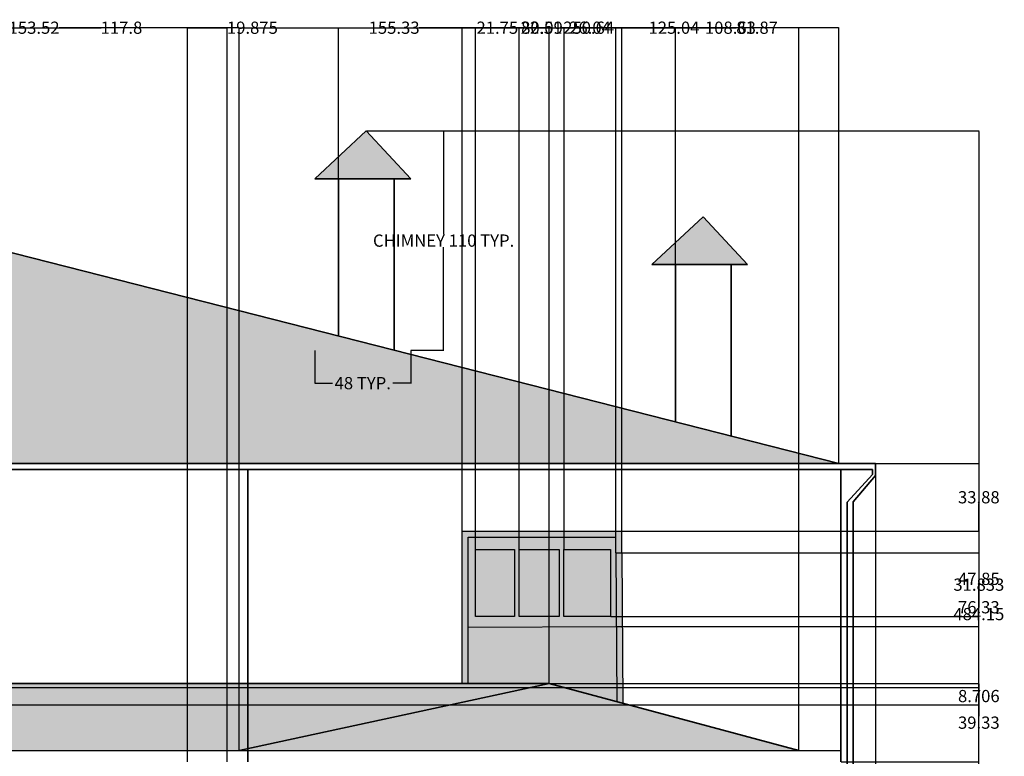
# Model space of a CAD drawing. Units: inches. Extents: x -655 to 499, y 20 to 616.
# Tile 7 of 7: x 5 to 499, y 246 to 616. Entities that reach past the tile are written whole.
import ezdxf

# ---------------------------------------------------------------- set-up
doc = ezdxf.new("R2010")
doc.units = ezdxf.units.IN
doc.header["$MEASUREMENT"] = 0
for name, color, linetype, lineweight in [('A-ANNO-DIMS', 2, 'Continuous', 18), ('A-ELEV', 7, 'Continuous', 35), ('A-ELEV-PATT', 9, 'Continuous', 13), ('A-GLAZ', 3, 'Continuous', 25), ('A-ROOF', 1, 'Continuous', 35)]:
    doc.layers.add(name, color=color, linetype=linetype, lineweight=lineweight)
doc.styles.get("Standard").update_dxf_attribs({"font": 'arial.ttf'})
doc.dimstyles.get("Standard").update_dxf_attribs({"dimtxt": 6.125, "dimasz": 0.18, "dimexe": 0.18, "dimexo": 0.0625, "dimgap": 0.09, "dimtad": 0, "dimtih": 1, "dimtoh": 1, "dimdec": 4, "dimzin": 0, "dimdsep": 46, "dimlunit": 4, "dimtxsty": 'Standard', "dimcen": 0.09, "dimadec": 0, "dimazin": 0, "dimtfac": 1, "dimtdec": 4, "dimtofl": 0, "dimtmove": 0, "dimatfit": 3, "dimfxl": 1, "dimtolj": 1, "dimtzin": 0, "dimarcsym": 0})

# ---------------------------------------------------------------- blocks, each defined once
blk = doc.blocks.new('CHIMNEY')
for p, q in [((25.81, 109.88), (0, 85.92)), ((25.81, 109.88), (48.05, 85.92)), ((0, 85.92), (11.86, 85.92)), ((11.86, 7.11), (11.86, 85.92)), ((39.76, 85.92), (11.86, 85.92)), ((39.76, 0), (39.76, 85.92)), ((48.05, 85.92), (39.76, 85.92))]:
    blk.add_line(p, q)
blk = doc.blocks.new('*D6')
at = {"layer": 'A-ANNO-DIMS', "color": 0, "lineweight": -2, "transparency": 16777216}
for p, q in [((201.35, 559.78), (217.95, 559.78)), ((217.77, 559.6), (217.77, 508.1)), ((217.77, 450.08), (217.77, 501.58)), ((201.35, 449.9), (217.95, 449.9))]:
    blk.add_line(p, q, dxfattribs=at)
at = {"layer": 'A-ANNO-DIMS', "color": 0, "transparency": 16777216}
for points in [[(217.74, 559.6), (217.8, 559.6), (217.77, 559.78)], [(217.74, 450.08), (217.8, 450.08), (217.77, 449.9)]]:
    blk.add_solid(points, dxfattribs=at)
at = {"layer": 'Defpoints', "color": 0, "transparency": 16777216}
for p in [(201.29, 559.78), (217.77, 559.78), (201.29, 449.9)]:
    blk.add_point(p, dxfattribs=at)
at = {"layer": 'A-ANNO-DIMS', "color": 0, "transparency": 16777216, "insert": (217.77, 504.84), "char_height": 6.125, "attachment_point": 5}
blk.add_mtext('\\A1;CHIMNEY 110 TYP.', dxfattribs=at)
blk = doc.blocks.new('*D7')
at = {"layer": 'A-ANNO-DIMS', "color": 0, "lineweight": -2, "transparency": 16777216}
for p, q in [((153.23, 449.84), (153.23, 433.24)), ((201.29, 449.84), (201.29, 433.24)), ((153.41, 433.42), (162.14, 433.42)), ((201.11, 433.42), (192.38, 433.42))]:
    blk.add_line(p, q, dxfattribs=at)
at = {"layer": 'A-ANNO-DIMS', "color": 0, "transparency": 16777216}
for points in [[(153.41, 433.45), (153.41, 433.39), (153.23, 433.42)], [(201.11, 433.45), (201.11, 433.39), (201.29, 433.42)]]:
    blk.add_solid(points, dxfattribs=at)
at = {"layer": 'Defpoints', "color": 0, "transparency": 16777216}
for p in [(153.23, 449.9), (201.29, 449.9), (201.29, 433.42)]:
    blk.add_point(p, dxfattribs=at)
at = {"layer": 'A-ANNO-DIMS', "color": 0, "transparency": 16777216, "insert": (177.26, 433.42), "char_height": 6.125, "attachment_point": 5}
blk.add_mtext('\\A1;48 TYP.', dxfattribs=at)
blk = doc.blocks.new('*D10')
at = {"layer": 'A-ANNO-DIMS', "color": 0, "lineweight": -2, "transparency": 16777216}
for p, q in [((434.11, 393.11), (434.11, 23.7)), ((-590.16, 75.57), (-590.16, 23.7)), ((-589.98, 23.88), (-90.54, 23.88)), ((433.93, 23.88), (-65.51, 23.88))]:
    blk.add_line(p, q, dxfattribs=at)
at = {"layer": 'A-ANNO-DIMS', "color": 0, "transparency": 16777216}
for points in [[(-589.98, 23.91), (-589.98, 23.85), (-590.16, 23.88)], [(433.93, 23.91), (433.93, 23.85), (434.11, 23.88)]]:
    blk.add_solid(points, dxfattribs=at)
at = {"layer": 'Defpoints', "color": 0, "transparency": 16777216}
for p in [(434.11, 393.17), (-590.16, 75.63), (434.11, 23.88)]:
    blk.add_point(p, dxfattribs=at)
at = {"layer": 'A-ANNO-DIMS', "color": 0, "transparency": 16777216, "insert": (-78.02, 23.88), "char_height": 6.125, "attachment_point": 5}
blk.add_mtext('\\A1;1024.3', dxfattribs=at)
blk = doc.blocks.new('*D18')
at = {"layer": 'A-ANNO-DIMS', "color": 0, "lineweight": -2, "transparency": 16777216}
for p, q in [((227.01, 359.35), (227.01, 611.71)), ((307.11, 359.35), (307.11, 611.71)), ((227.19, 611.53), (256.63, 611.53)), ((306.93, 611.53), (277.49, 611.53))]:
    blk.add_line(p, q, dxfattribs=at)
at = {"layer": 'A-ANNO-DIMS', "color": 0, "transparency": 16777216}
for points in [[(227.19, 611.56), (227.19, 611.5), (227.01, 611.53)], [(306.93, 611.56), (306.93, 611.5), (307.11, 611.53)]]:
    blk.add_solid(points, dxfattribs=at)
at = {"layer": 'Defpoints', "color": 0, "transparency": 16777216}
for p in [(307.11, 611.53), (227.01, 359.29), (307.11, 359.29)]:
    blk.add_point(p, dxfattribs=at)
at = {"layer": 'A-ANNO-DIMS', "color": 0, "transparency": 16777216, "insert": (267.06, 611.53), "char_height": 6.125, "attachment_point": 5}
blk.add_mtext('\\A1;80.09', dxfattribs=at)
blk = doc.blocks.new('*D19')
at = {"layer": 'A-ANNO-DIMS', "color": 0, "lineweight": -2, "transparency": 16777216}
for p, q in [((165.1, 457.07), (165.1, 611.71)), ((415.74, 393.23), (415.74, 611.71)), ((165.28, 611.53), (277.57, 611.53)), ((415.56, 611.53), (303.26, 611.53))]:
    blk.add_line(p, q, dxfattribs=at)
at = {"layer": 'A-ANNO-DIMS', "color": 0, "transparency": 16777216}
for points in [[(165.28, 611.56), (165.28, 611.5), (165.1, 611.53)], [(415.56, 611.56), (415.56, 611.5), (415.74, 611.53)]]:
    blk.add_solid(points, dxfattribs=at)
at = {"layer": 'Defpoints', "color": 0, "transparency": 16777216}
for p in [(415.74, 611.53), (165.1, 457), (415.74, 393.17)]:
    blk.add_point(p, dxfattribs=at)
at = {"layer": 'A-ANNO-DIMS', "color": 0, "transparency": 16777216, "insert": (290.42, 611.53), "char_height": 6.125, "attachment_point": 5}
blk.add_mtext('\\A1;250.64', dxfattribs=at)
blk = doc.blocks.new('*D20')
at = {"layer": 'A-ANNO-DIMS', "color": 0, "lineweight": -2, "transparency": 16777216}
for p, q in [((333.87, 414.08), (333.87, 611.71)), ((415.74, 393.23), (415.74, 611.71)), ((334.05, 611.53), (364.37, 611.53)), ((415.56, 611.53), (385.23, 611.53))]:
    blk.add_line(p, q, dxfattribs=at)
at = {"layer": 'A-ANNO-DIMS', "color": 0, "transparency": 16777216}
for points in [[(334.05, 611.56), (334.05, 611.5), (333.87, 611.53)], [(415.56, 611.56), (415.56, 611.5), (415.74, 611.53)]]:
    blk.add_solid(points, dxfattribs=at)
at = {"layer": 'Defpoints', "color": 0, "transparency": 16777216}
for p in [(415.74, 611.53), (333.87, 414.02), (415.74, 393.17)]:
    blk.add_point(p, dxfattribs=at)
at = {"layer": 'A-ANNO-DIMS', "color": 0, "transparency": 16777216, "insert": (374.8, 611.53), "char_height": 6.125, "attachment_point": 5}
blk.add_mtext('\\A1;81.87', dxfattribs=at)
blk = doc.blocks.new('*D21')
at = {"layer": 'A-ANNO-DIMS', "color": 0, "lineweight": -2, "transparency": 16777216}
for p, q in [((179.11, 559.78), (486.04, 559.78)), ((485.86, 559.6), (485.86, 320.92)), ((485.86, 75.81), (485.86, 314.49)), ((-590.1, 75.63), (486.04, 75.63))]:
    blk.add_line(p, q, dxfattribs=at)
at = {"layer": 'A-ANNO-DIMS', "color": 0, "transparency": 16777216}
for points in [[(485.83, 559.6), (485.89, 559.6), (485.86, 559.78)], [(485.83, 75.81), (485.89, 75.81), (485.86, 75.63)]]:
    blk.add_solid(points, dxfattribs=at)
at = {"layer": 'Defpoints', "color": 0, "transparency": 16777216}
for p in [(179.05, 559.78), (485.86, 559.78), (-590.16, 75.63)]:
    blk.add_point(p, dxfattribs=at)
at = {"layer": 'A-ANNO-DIMS', "color": 0, "transparency": 16777216, "insert": (485.86, 317.7), "char_height": 6.125, "attachment_point": 5}
blk.add_mtext('\\A1;484.15', dxfattribs=at)
blk = doc.blocks.new('*D35')
at = {"layer": 'A-ANNO-DIMS', "color": 0, "lineweight": -2, "transparency": 16777216}
for p, q in [((-244.62, 280.97), (486.04, 280.97)), ((485.86, 280.79), (485.86, 279.83)), ((-226.95, 272.26), (486.04, 272.26)), ((485.86, 272.44), (485.86, 273.4))]:
    blk.add_line(p, q, dxfattribs=at)
at = {"layer": 'A-ANNO-DIMS', "color": 0, "transparency": 16777216}
for points in [[(485.83, 280.79), (485.89, 280.79), (485.86, 280.97)], [(485.83, 272.44), (485.89, 272.44), (485.86, 272.26)]]:
    blk.add_solid(points, dxfattribs=at)
at = {"layer": 'Defpoints', "color": 0, "transparency": 16777216}
for p in [(-244.69, 280.97), (-227.01, 272.26), (485.86, 272.26)]:
    blk.add_point(p, dxfattribs=at)
at = {"layer": 'A-ANNO-DIMS', "color": 0, "transparency": 16777216, "insert": (485.86, 276.61), "char_height": 6.125, "attachment_point": 5}
blk.add_mtext('\\A1;8.706', dxfattribs=at)
blk = doc.blocks.new('*D56')
at = {"layer": 'A-ANNO-DIMS', "color": 0, "lineweight": -2, "transparency": 16777216}
for p, q in [((-2.5, 283.02), (-2.5, 611.71)), ((115.31, 249.31), (115.31, 611.71)), ((-2.32, 611.53), (46.26, 611.53)), ((115.13, 611.53), (66.55, 611.53))]:
    blk.add_line(p, q, dxfattribs=at)
at = {"layer": 'A-ANNO-DIMS', "color": 0, "transparency": 16777216}
for points in [[(-2.32, 611.56), (-2.32, 611.5), (-2.5, 611.53)], [(115.13, 611.56), (115.13, 611.5), (115.31, 611.53)]]:
    blk.add_solid(points, dxfattribs=at)
at = {"layer": 'Defpoints', "color": 0, "transparency": 16777216}
for p in [(115.31, 611.53), (-2.5, 282.96), (115.31, 249.25)]:
    blk.add_point(p, dxfattribs=at)
at = {"layer": 'A-ANNO-DIMS', "color": 0, "transparency": 16777216, "insert": (56.41, 611.53), "char_height": 6.125, "attachment_point": 5}
blk.add_mtext('\\A1;117.8', dxfattribs=at)
blk = doc.blocks.new('*D57')
at = {"layer": 'A-ANNO-DIMS', "color": 0, "lineweight": -2, "transparency": 16777216}
for p, q in [((115.31, 249.31), (115.31, 611.71)), ((270.64, 283.02), (270.64, 611.71)), ((115.49, 611.53), (180.46, 611.53)), ((270.46, 611.53), (205.49, 611.53))]:
    blk.add_line(p, q, dxfattribs=at)
at = {"layer": 'A-ANNO-DIMS', "color": 0, "transparency": 16777216}
for points in [[(115.49, 611.56), (115.49, 611.5), (115.31, 611.53)], [(270.46, 611.56), (270.46, 611.5), (270.64, 611.53)]]:
    blk.add_solid(points, dxfattribs=at)
at = {"layer": 'Defpoints', "color": 0, "transparency": 16777216}
for p in [(270.64, 611.53), (270.64, 282.96), (115.31, 249.25)]:
    blk.add_point(p, dxfattribs=at)
at = {"layer": 'A-ANNO-DIMS', "color": 0, "transparency": 16777216, "insert": (192.97, 611.53), "char_height": 6.125, "attachment_point": 5}
blk.add_mtext('\\A1;155.33', dxfattribs=at)
blk = doc.blocks.new('*D58')
at = {"layer": 'A-ANNO-DIMS', "color": 0, "lineweight": -2, "transparency": 16777216}
for p, q in [((270.64, 283.02), (270.64, 611.71)), ((395.67, 249.37), (395.67, 611.71)), ((270.82, 611.53), (320.65, 611.53)), ((395.49, 611.53), (345.66, 611.53))]:
    blk.add_line(p, q, dxfattribs=at)
at = {"layer": 'A-ANNO-DIMS', "color": 0, "transparency": 16777216}
for points in [[(270.82, 611.56), (270.82, 611.5), (270.64, 611.53)], [(395.49, 611.56), (395.49, 611.5), (395.67, 611.53)]]:
    blk.add_solid(points, dxfattribs=at)
at = {"layer": 'Defpoints', "color": 0, "transparency": 16777216}
for p in [(395.67, 611.53), (270.64, 282.96), (395.67, 249.31)]:
    blk.add_point(p, dxfattribs=at)
at = {"layer": 'A-ANNO-DIMS', "color": 0, "transparency": 16777216, "insert": (333.16, 611.53), "char_height": 6.125, "attachment_point": 5}
blk.add_mtext('\\A1;125.04', dxfattribs=at)
blk = doc.blocks.new('*D61')
at = {"layer": 'A-ANNO-DIMS', "color": 0, "lineweight": -2, "transparency": 16777216}
for p, q in [((-64.12, 233.34), (-64.12, 611.71)), ((89.4, 243.69), (89.4, 611.71)), ((-63.94, 611.53), (0.16, 611.53)), ((89.22, 611.53), (25.13, 611.53))]:
    blk.add_line(p, q, dxfattribs=at)
at = {"layer": 'A-ANNO-DIMS', "color": 0, "transparency": 16777216}
for points in [[(-63.94, 611.56), (-63.94, 611.5), (-64.12, 611.53)], [(89.22, 611.56), (89.22, 611.5), (89.4, 611.53)]]:
    blk.add_solid(points, dxfattribs=at)
at = {"layer": 'Defpoints', "color": 0, "transparency": 16777216}
for p in [(89.4, 611.53), (89.4, 243.63), (-64.12, 233.27)]:
    blk.add_point(p, dxfattribs=at)
at = {"layer": 'A-ANNO-DIMS', "color": 0, "transparency": 16777216, "insert": (12.64, 611.53), "char_height": 6.125, "attachment_point": 5}
blk.add_mtext('\\A1;153.52', dxfattribs=at)
blk = doc.blocks.new('*D62')
at = {"layer": 'A-ANNO-DIMS', "color": 0, "lineweight": -2, "transparency": 16777216}
for p, q in [((89.4, 243.69), (89.4, 611.71)), ((109.28, 243.69), (109.28, 611.71)), ((89.58, 611.53), (109.1, 611.53)), ((109.28, 611.53), (109.46, 611.53))]:
    blk.add_line(p, q, dxfattribs=at)
at = {"layer": 'A-ANNO-DIMS', "color": 0, "transparency": 16777216}
for points in [[(89.58, 611.56), (89.58, 611.5), (89.4, 611.53)], [(109.1, 611.56), (109.1, 611.5), (109.28, 611.53)]]:
    blk.add_solid(points, dxfattribs=at)
at = {"layer": 'Defpoints', "color": 0, "transparency": 16777216}
for p in [(109.28, 611.53), (89.4, 243.63), (109.28, 243.63)]:
    blk.add_point(p, dxfattribs=at)
at = {"layer": 'A-ANNO-DIMS', "color": 0, "transparency": 16777216, "insert": (121.99, 611.53), "char_height": 6.125, "attachment_point": 5}
blk.add_mtext('\\A1;19.875', dxfattribs=at)
blk = doc.blocks.new('*D80')
at = {"layer": 'A-ANNO-DIMS', "color": 0, "lineweight": -2, "transparency": 16777216}
for p, q in [((270.7, 282.96), (486.04, 282.96)), ((485.86, 282.78), (485.86, 266.51)), ((485.86, 243.81), (485.86, 260.07)), ((416.84, 243.63), (486.04, 243.63))]:
    blk.add_line(p, q, dxfattribs=at)
at = {"layer": 'A-ANNO-DIMS', "color": 0, "transparency": 16777216}
for points in [[(485.83, 282.78), (485.89, 282.78), (485.86, 282.96)], [(485.83, 243.81), (485.89, 243.81), (485.86, 243.63)]]:
    blk.add_solid(points, dxfattribs=at)
at = {"layer": 'Defpoints', "color": 0, "transparency": 16777216}
for p in [(270.64, 282.96), (485.86, 282.96), (416.78, 243.63)]:
    blk.add_point(p, dxfattribs=at)
at = {"layer": 'A-ANNO-DIMS', "color": 0, "transparency": 16777216, "insert": (485.86, 263.29), "char_height": 6.125, "attachment_point": 5}
blk.add_mtext('\\A1;39.33', dxfattribs=at)
blk = doc.blocks.new('*D81')
at = {"layer": 'A-ANNO-DIMS', "color": 0, "lineweight": -2, "transparency": 16777216}
for p, q in [((307.17, 359.29), (486.04, 359.29)), ((485.86, 359.11), (485.86, 324.34)), ((485.86, 283.14), (485.86, 317.9)), ((270.7, 282.96), (486.04, 282.96))]:
    blk.add_line(p, q, dxfattribs=at)
at = {"layer": 'A-ANNO-DIMS', "color": 0, "transparency": 16777216}
for points in [[(485.83, 359.11), (485.89, 359.11), (485.86, 359.29)], [(485.83, 283.14), (485.89, 283.14), (485.86, 282.96)]]:
    blk.add_solid(points, dxfattribs=at)
at = {"layer": 'Defpoints', "color": 0, "transparency": 16777216}
for p in [(307.11, 359.29), (485.86, 359.29), (270.64, 282.96)]:
    blk.add_point(p, dxfattribs=at)
at = {"layer": 'A-ANNO-DIMS', "color": 0, "transparency": 16777216, "insert": (485.86, 321.12), "char_height": 6.125, "attachment_point": 5}
blk.add_mtext('\\A1;76.33', dxfattribs=at)
blk = doc.blocks.new('*D82')
at = {"layer": 'A-ANNO-DIMS', "color": 0, "lineweight": -2, "transparency": 16777216}
for p, q in [((415.8, 393.17), (486.04, 393.17)), ((485.86, 392.99), (485.86, 379.44)), ((485.86, 359.47), (485.86, 373.01)), ((307.17, 359.29), (486.04, 359.29))]:
    blk.add_line(p, q, dxfattribs=at)
at = {"layer": 'A-ANNO-DIMS', "color": 0, "transparency": 16777216}
for points in [[(485.83, 392.99), (485.89, 392.99), (485.86, 393.17)], [(485.83, 359.47), (485.89, 359.47), (485.86, 359.29)]]:
    blk.add_solid(points, dxfattribs=at)
at = {"layer": 'Defpoints', "color": 0, "transparency": 16777216}
for p in [(415.74, 393.17), (485.86, 393.17), (307.11, 359.29)]:
    blk.add_point(p, dxfattribs=at)
at = {"layer": 'A-ANNO-DIMS', "color": 0, "transparency": 16777216, "insert": (485.86, 376.23), "char_height": 6.125, "attachment_point": 5}
blk.add_mtext('\\A1;33.88', dxfattribs=at)
blk = doc.blocks.new('*D83')
at = {"layer": 'A-ANNO-DIMS', "color": 0, "lineweight": -2, "transparency": 16777216}
for p, q in [((307.17, 359.29), (486.04, 359.29)), ((485.86, 359.11), (485.86, 338.58)), ((485.86, 311.62), (485.86, 332.14)), ((304.35, 311.44), (486.04, 311.44))]:
    blk.add_line(p, q, dxfattribs=at)
at = {"layer": 'A-ANNO-DIMS', "color": 0, "transparency": 16777216}
for points in [[(485.83, 359.11), (485.89, 359.11), (485.86, 359.29)], [(485.83, 311.62), (485.89, 311.62), (485.86, 311.44)]]:
    blk.add_solid(points, dxfattribs=at)
at = {"layer": 'Defpoints', "color": 0, "transparency": 16777216}
for p in [(307.11, 359.29), (485.86, 359.29), (304.28, 311.44)]:
    blk.add_point(p, dxfattribs=at)
at = {"layer": 'A-ANNO-DIMS', "color": 0, "transparency": 16777216, "insert": (485.86, 335.36), "char_height": 6.125, "attachment_point": 5}
blk.add_mtext('\\A1;47.85', dxfattribs=at)
blk = doc.blocks.new('*D84')
at = {"layer": 'A-ANNO-DIMS', "color": 0, "lineweight": -2, "transparency": 16777216}
for p, q in [((304.17, 348.34), (486.04, 348.34)), ((485.86, 348.16), (485.86, 335.65)), ((485.86, 316.69), (485.86, 329.21)), ((301.47, 316.51), (486.04, 316.51))]:
    blk.add_line(p, q, dxfattribs=at)
at = {"layer": 'A-ANNO-DIMS', "color": 0, "transparency": 16777216}
for points in [[(485.83, 348.16), (485.89, 348.16), (485.86, 348.34)], [(485.83, 316.69), (485.89, 316.69), (485.86, 316.51)]]:
    blk.add_solid(points, dxfattribs=at)
at = {"layer": 'Defpoints', "color": 0, "transparency": 16777216}
for p in [(304.11, 348.34), (485.86, 348.34), (301.41, 316.51)]:
    blk.add_point(p, dxfattribs=at)
at = {"layer": 'A-ANNO-DIMS', "color": 0, "transparency": 16777216, "insert": (485.86, 332.43), "char_height": 6.125, "attachment_point": 5}
blk.add_mtext('\\A1;31.833', dxfattribs=at)
blk = doc.blocks.new('*D85')
at = {"layer": 'A-ANNO-DIMS', "color": 0, "lineweight": -2, "transparency": 16777216}
for p, q in [((307.11, 359.35), (307.11, 611.71)), ((415.74, 393.23), (415.74, 611.71)), ((307.29, 611.53), (348.91, 611.53)), ((415.56, 611.53), (373.94, 611.53))]:
    blk.add_line(p, q, dxfattribs=at)
at = {"layer": 'A-ANNO-DIMS', "color": 0, "transparency": 16777216}
for points in [[(307.29, 611.56), (307.29, 611.5), (307.11, 611.53)], [(415.56, 611.56), (415.56, 611.5), (415.74, 611.53)]]:
    blk.add_solid(points, dxfattribs=at)
at = {"layer": 'Defpoints', "color": 0, "transparency": 16777216}
for p in [(415.74, 611.53), (415.74, 393.17), (307.11, 359.29)]:
    blk.add_point(p, dxfattribs=at)
at = {"layer": 'A-ANNO-DIMS', "color": 0, "transparency": 16777216, "insert": (361.42, 611.53), "char_height": 6.125, "attachment_point": 5}
blk.add_mtext('\\A1;108.63', dxfattribs=at)
blk = doc.blocks.new('*D86')
at = {"layer": 'A-ANNO-DIMS', "color": 0, "lineweight": -2, "transparency": 16777216}
for p, q in [((233.81, 350.08), (233.81, 611.71)), ((255.56, 350.08), (255.56, 611.71)), ((233.99, 611.53), (234.19, 611.53)), ((255.38, 611.53), (255.18, 611.53))]:
    blk.add_line(p, q, dxfattribs=at)
at = {"layer": 'A-ANNO-DIMS', "color": 0, "transparency": 16777216}
for points in [[(233.99, 611.56), (233.99, 611.5), (233.81, 611.53)], [(255.38, 611.56), (255.38, 611.5), (255.56, 611.53)]]:
    blk.add_solid(points, dxfattribs=at)
at = {"layer": 'Defpoints', "color": 0, "transparency": 16777216}
for p in [(255.56, 611.53), (233.81, 350.02), (255.56, 350.02)]:
    blk.add_point(p, dxfattribs=at)
at = {"layer": 'A-ANNO-DIMS', "color": 0, "transparency": 16777216, "insert": (244.68, 611.53), "char_height": 6.125, "attachment_point": 5}
blk.add_mtext('\\A1;21.75', dxfattribs=at)
blk = doc.blocks.new('*D87')
at = {"layer": 'A-ANNO-DIMS', "color": 0, "lineweight": -2, "transparency": 16777216}
for p, q in [((255.56, 350.08), (255.56, 611.71)), ((278.07, 350.08), (278.07, 611.71)), ((255.74, 611.53), (256.93, 611.53)), ((277.89, 611.53), (276.7, 611.53))]:
    blk.add_line(p, q, dxfattribs=at)
at = {"layer": 'A-ANNO-DIMS', "color": 0, "transparency": 16777216}
for points in [[(255.74, 611.56), (255.74, 611.5), (255.56, 611.53)], [(277.89, 611.56), (277.89, 611.5), (278.07, 611.53)]]:
    blk.add_solid(points, dxfattribs=at)
at = {"layer": 'Defpoints', "color": 0, "transparency": 16777216}
for p in [(278.07, 611.53), (255.56, 350.02), (278.07, 350.02)]:
    blk.add_point(p, dxfattribs=at)
at = {"layer": 'A-ANNO-DIMS', "color": 0, "transparency": 16777216, "insert": (266.81, 611.53), "char_height": 6.125, "attachment_point": 5}
blk.add_mtext('\\A1;22.51', dxfattribs=at)
blk = doc.blocks.new('*D88')
at = {"layer": 'A-ANNO-DIMS', "color": 0, "lineweight": -2, "transparency": 16777216}
for p, q in [((278.07, 350.08), (278.07, 611.71)), ((304.11, 348.41), (304.11, 611.71)), ((278.25, 611.53), (280.62, 611.53)), ((303.93, 611.53), (301.55, 611.53))]:
    blk.add_line(p, q, dxfattribs=at)
at = {"layer": 'A-ANNO-DIMS', "color": 0, "transparency": 16777216}
for points in [[(278.25, 611.56), (278.25, 611.5), (278.07, 611.53)], [(303.93, 611.56), (303.93, 611.5), (304.11, 611.53)]]:
    blk.add_solid(points, dxfattribs=at)
at = {"layer": 'Defpoints', "color": 0, "transparency": 16777216}
for p in [(304.11, 611.53), (278.07, 350.02), (304.11, 348.34)]:
    blk.add_point(p, dxfattribs=at)
at = {"layer": 'A-ANNO-DIMS', "color": 0, "transparency": 16777216, "insert": (291.09, 611.53), "char_height": 6.125, "attachment_point": 5}
blk.add_mtext('\\A1;26.04', dxfattribs=at)

msp = doc.modelspace()

# ---------------------------------------------------------------- hatches: boundary and pattern name
at = {"layer": 'A-ELEV-PATT'}
h = msp.add_hatch(color=256, dxfattribs=at)
h.dxf.hatch_style = 1
h.paths.add_polyline_path([(-140.0489, 272.2618), (-399.3758, 272.2618), (-399.3758, 249.8418), (-399.3758, 248.5179), (-366.9446, 248.7444), (-209.8047, 249.8418), (-183.5755, 249.8418), (-140.0489, 249.8418)])
h.paths.add_polyline_path([(-211.7589, 317.0515), (-216.5713, 317.0515), (-216.5713, 272.2618), (-211.7589, 272.2618)])
h.paths.add_polyline_path([(-145.96, 317.0515), (-150.7725, 317.0515), (-150.7725, 272.2618), (-145.96, 272.2618)])
h.paths.add_polyline_path([(-140.5198, 321.4867), (-402.0739, 321.4867), (-402.0739, 317.0515), (-390.1757, 317.0515), (-385.3633, 317.0515), (-150.7725, 317.0515), (-145.96, 317.0515), (-140.5198, 317.0515)])
h.paths.add_polyline_path([(-269.7123, 317.0515), (-274.5248, 317.0515), (-274.5248, 272.2618), (-269.7123, 272.2618)])
h.paths.add_polyline_path([(-329.7837, 317.0515), (-334.5961, 317.0515), (-334.5961, 280.9678), (-329.7837, 280.9678)])
h.paths.add_polyline_path([(-329.7837, 280.9678), (-334.5961, 280.9678), (-334.5961, 272.2618), (-329.7837, 272.2618)])
h.paths.add_polyline_path([(-385.3633, 317.0515), (-390.1757, 317.0515), (-390.1757, 272.2618), (-385.3633, 272.2618)])
h.paths.add_polyline_path([(-229.0087, 240.4184), (-354.3532, 240.4184), (-354.2854, 210.6425), (-315.9956, 210.6425), (-315.9956, 210.9348), (-277.6793, 210.7995), (-277.6793, 210.6425), (-273.1052, 210.6425), (-273.1052, 210.7995), (-229.3637, 210.6425), (-229.0087, 210.6425)])
h.paths.add_polyline_path([(-229.0087, 145.8007), (-354.3532, 145.8007), (-354.3532, 101.6296), (-229.0087, 101.6296)])
h.paths.add_polyline_path([(-229.0087, 210.6425), (-229.3637, 210.6425), (-229.3637, 151.3385), (-273.1052, 151.4955), (-273.1052, 210.6425), (-277.6793, 210.6425), (-277.6793, 151.4955), (-315.9956, 151.6308), (-315.9956, 210.6425), (-318.9742, 210.6425), (-318.9742, 151.3385), (-354.3532, 151.3385), (-354.3532, 145.8007), (-229.0087, 145.8007)])
h.paths.add_polyline_path([(-229.0087, 247.8418), (-354.3532, 247.8418), (-354.3532, 240.4184), (-229.0087, 240.4184)])
h.paths.add_polyline_path([(4.4271, 93.6296), (-100.4134, 93.6296), (-124.8077, 93.6296), (-126.8077, 93.6296), (-126.8077, 87.6296), (4.4271, 87.6296)])
h.paths.add_polyline_path([(4.4271, 99.6296), (-100.4134, 99.6296), (-100.4134, 93.6296), (4.4271, 93.6296)])
h.paths.add_polyline_path([(99.4982, 99.6296), (6.4271, 99.6296), (6.4271, 93.6296), (99.4982, 93.6296)])
h.paths.add_polyline_path([(99.4982, 93.6296), (6.4271, 93.6296), (6.4271, 87.6296), (99.4982, 87.6296)])
h.paths.add_polyline_path([(304.2843, 311.436), (230.0144, 311.076), (230.0144, 282.9577), (270.6361, 282.9577), (304.4665, 273.8535)])
h.paths.add_polyline_path([(304.1054, 348.3371), (304.1054, 356.2861), (230.0144, 356.2861), (230.0144, 348.3443), (230.0144, 311.076), (304.2843, 311.436)])
h.paths.add_polyline_path([(255.5586, 316.5111), (255.5586, 350.0185), (275.6848, 350.0185), (275.6848, 316.5111)], flags=16)
h.paths.add_polyline_path([(278.0676, 316.5111), (278.0676, 350.0185), (301.4074, 350.0185), (301.4074, 316.5111)], flags=16)
h.paths.add_polyline_path([(253.2029, 316.5111), (233.8107, 316.5111), (233.8107, 350.0185), (253.2029, 350.0185)], flags=16)
h.paths.add_polyline_path([(179.0482, 559.7795), (153.2347, 535.8185), (165.0976, 535.8185), (192.9989, 535.8185), (201.2897, 535.8185)])
h.paths.add_polyline_path([(347.8163, 516.7932), (322.0028, 492.8322), (333.8657, 492.8322), (361.7669, 492.8322), (370.0577, 492.8322)])
h = msp.add_hatch(color=256, dxfattribs=at)
h.dxf.hatch_style = 1
h.paths.add_polyline_path([(-209.8047, 249.8418), (-366.9446, 248.7444), (-366.9446, 98.5321), (-209.8047, 99.6296)])
h.paths.add_polyline_path([(-229.0087, 101.6296), (-354.3532, 101.6296), (-354.3532, 247.8418), (-229.0087, 247.8418), (-229.0087, 240.4184), (-228.941, 210.6425), (-229.0087, 210.6425)], flags=16)
h.paths.add_polyline_path([(-229.3637, 151.3385), (-273.1052, 151.4955), (-273.1052, 210.7995), (-229.3637, 210.6425)], flags=0)
h.paths.add_polyline_path([(-277.6793, 151.4955), (-315.9956, 151.6308), (-315.9956, 210.9348), (-277.6793, 210.7995)], flags=0)
h.paths.add_polyline_path([(-318.9742, 151.3385), (-354.3532, 151.3385), (-354.3532, 210.6425), (-318.9742, 210.6425)], flags=0)
h.paths.add_polyline_path([(230.0144, 348.3443), (230.0144, 356.2861), (304.1054, 356.2861), (304.1054, 348.3371), (304.4665, 273.8535), (307.4704, 273.0451), (307.1054, 348.3443), (307.1054, 359.2861), (227.0144, 359.2861), (227.0144, 348.3443), (227.0144, 282.9577), (230.0144, 282.9577)])
h = msp.add_hatch(color=256, dxfattribs=at)
h.dxf.hatch_style = 1
h.paths.add_polyline_path([(-329.7837, 350.1333), (-347.0336, 350.1333), (-347.0336, 321.4867), (-329.7837, 321.4867)])
h.paths.add_polyline_path([(-294.1413, 350.1333), (-311.3912, 350.1333), (-311.3912, 321.4867), (-294.1413, 321.4867)])
h.paths.add_polyline_path([(-294.1413, 317.0515), (-311.3912, 317.0515), (-311.3912, 280.9678), (-294.1413, 280.9678)])
h.paths.add_polyline_path([(-334.5961, 317.0515), (-347.0336, 317.0515), (-347.0336, 280.9678), (-334.5961, 280.9678)])
h.paths.add_polyline_path([(-244.6859, 336.719), (-258.4486, 336.719), (-258.4486, 347.0139), (-244.6859, 347.0139), (-244.6859, 350.1333), (-261.9358, 350.1333), (-261.9358, 321.4867), (-244.6859, 321.4867)])
h.paths.add_polyline_path([(-244.6859, 317.0515), (-261.9358, 317.0515), (-261.9358, 280.9678), (-244.6859, 280.9678)])
h.paths.add_polyline_path([(-244.6859, 347.0139), (-258.4486, 347.0139), (-258.4486, 336.719), (-244.6859, 336.719)], flags=17)
h.paths.add_polyline_path([(-318.9742, 210.6425), (-354.3532, 210.6425), (-354.3532, 151.3385), (-318.9742, 151.3385)])
h.paths.add_polyline_path([(-277.6793, 210.6425), (-315.9956, 210.6425), (-315.9956, 151.6308), (-277.6793, 151.4955)])
h.paths.add_polyline_path([(-229.3637, 210.6425), (-273.1052, 210.6425), (-273.1052, 151.4955), (-229.3637, 151.3385)])
h.paths.add_polyline_path([(-19.537, 192.4712), (-40.2951, 192.4712), (-40.2951, 150.3082), (-19.537, 150.3082)])
h.paths.add_polyline_path([(2.4271, 231.274), (-62.1158, 231.274), (-62.1158, 210.7923), (2.4271, 210.7923)])
h.paths.add_polyline_path([(72.97, 231.274), (8.4271, 231.274), (8.4271, 210.7923), (72.97, 210.7923)])
h.paths.add_polyline_path([(51.0059, 192.4712), (30.2478, 192.4712), (30.2478, 150.3082), (51.0059, 150.3082)])
h.paths.add_polyline_path([(51.0059, 132.6671), (30.2478, 132.6671), (30.2478, 112.5254), (51.0059, 112.5254)])
h.paths.add_polyline_path([(-19.537, 132.6671), (-40.2951, 132.6671), (-40.2951, 112.5254), (-19.537, 112.5254)])
h.paths.add_polyline_path([(275.6848, 350.0185), (255.5586, 350.0185), (255.5586, 316.5111), (275.6848, 316.5111)])
h.paths.add_polyline_path([(301.4074, 350.0185), (278.0676, 350.0185), (278.0676, 316.5111), (301.4074, 316.5111)])
h.paths.add_polyline_path([(253.2029, 350.0185), (233.8107, 350.0185), (233.8107, 316.5111), (253.2029, 316.5111)])
at = {"layer": 'A-ROOF'}
h = msp.add_hatch(dxfattribs=at)
h.set_pattern_fill('AR-RSHKE', color=256)
h.paths.add_polyline_path([(-5.7434, 500.5192), (-493.0344, 393.1054), (-371.042, 393.1054), (119.6374, 393.1054), (415.7378, 393.1651)])
h.paths.add_polyline_path([(119.638, 282.9577), (-2.4978, 282.9577), (-133.531, 249.2017), (115.3098, 249.2518), (119.638, 250.1911)])
h.paths.add_polyline_path([(270.6361, 282.9577), (119.638, 282.9577), (119.638, 250.1911)], flags=17)
h.paths.add_polyline_path([(270.6361, 282.9577), (119.638, 250.1911), (119.638, 249.2527), (395.6741, 249.3083)])
h.paths.add_polyline_path([(-493.0344, 269.4313), (-534.9108, 229.7008), (-493.0344, 229.7008)])

# ---------------------------------------------------------------- linework, layer by layer
at = {"layer": 'A-ELEV'}
for p, q in [((416.7758, 243.6296), (416.7463, 390.1653)), ((119.638, 243.6296), (119.638, 387.6296)), ((419.8436, 99.6296), (419.8436, 373.8555)), ((422.8436, 99.6296), (422.8436, 373.8964))]:
    msp.add_line(p, q, dxfattribs=at)
at = {"layer": 'A-GLAZ'}
for p, q in [((227.0144, 359.2861), (307.1054, 359.2861)), ((227.0144, 348.3443), (227.0144, 359.2861)), ((230.0144, 356.2861), (304.1054, 356.2861)), ((230.0144, 348.3443), (230.0144, 356.2861)), ((304.1054, 348.3443), (304.1054, 356.2861)), ((307.1054, 348.3443), (307.1054, 359.2861)), ((227.0144, 282.9577), (227.0144, 348.3443)), ((230.0144, 282.9577), (230.0144, 348.3443)), ((304.1055, 348.3298), (304.4665, 273.8535)), ((307.1054, 348.3443), (307.4704, 273.0451)), ((230.0144, 311.076), (304.2843, 311.436))]:
    msp.add_line(p, q, dxfattribs=at)
for points in [[(233.8107, 350.0185), (253.2029, 350.0185), (253.2029, 316.5111), (233.8107, 316.5111)], [(255.5586, 350.0185), (275.6848, 350.0185), (275.6848, 316.5111), (255.5586, 316.5111)], [(278.0676, 350.0185), (301.4074, 350.0185), (301.4074, 316.5111), (278.0676, 316.5111)]]:
    msp.add_lwpolyline(points, close=True, dxfattribs=at)
at = {"layer": 'A-ROOF'}
for p, q in [((-5.7434, 500.5192), (415.7378, 393.1651)), ((119.6375, 390.1054), (-322.5736, 390.1054)), ((119.638, 387.6296), (119.6375, 390.1054)), ((119.638, 390.1054), (432.6079, 390.1685)), ((434.1137, 393.1688), (432.6073, 393.1685)), ((432.6079, 387.6927), (432.6079, 390.1685)), ((434.1137, 390.1685), (434.1137, 393.1688)), ((434.1137, 387.1304), (434.1137, 390.1685)), ((419.8436, 373.8555), (432.6079, 387.6927)), ((422.8436, 373.8964), (434.1137, 387.1304)), ((-2.4978, 282.9577), (270.6361, 282.9577)), ((115.3098, 249.2518), (270.6361, 282.9577)), ((270.6361, 282.9577), (395.6741, 249.3083)), ((-133.531, 249.2017), (416.7746, 249.3126))]:
    msp.add_line(p, q, dxfattribs=at)
msp.add_lwpolyline([(432.6073, 393.1685), (119.6374, 393.1054), (-371.042, 393.1054), (-493.0344, 393.1054)], dxfattribs=at)

# ---------------------------------------------------------------- block references
for p in [(153.235, 449.898), (322.003, 406.9117)]:
    msp.add_blockref('CHIMNEY', p, dxfattribs=at)

# ---------------------------------------------------------------- dimensions: what is measured, and where the dimension line sits
at = {"layer": 'A-ANNO-DIMS'}
for base, p1, p2, override, picture, middle in [((89.4008, 611.5295), (-64.1158, 233.274), (89.4008, 243.6296), {"dimdec": 2, "dimlfac": 1, "dimrnd": 0, "dimzin": 0, "dimdsep": 46, "dimlunit": 2}, '*D61', (12.6425, 611.5295)), ((115.3098, 611.5295), (-2.4978, 282.9577), (115.3098, 249.2518), {"dimdec": 1, "dimlfac": 1, "dimrnd": 0, "dimzin": 0, "dimdsep": 46, "dimlunit": 2}, '*D56', (56.406, 611.5295)), ((109.27634, 611.52951), (89.40085, 243.6296), (109.27634, 243.6296), {"dimdec": 3, "dimlfac": 1, "dimrnd": 0, "dimzin": 0, "dimdsep": 46, "dimlunit": 2}, '*D62', (121.99479, 611.52951)), ((270.6361, 611.5295), (115.3098, 249.2518), (270.6361, 282.9577), {"dimdec": 2, "dimlfac": 1, "dimrnd": 0, "dimzin": 0, "dimdsep": 46, "dimlunit": 2}, '*D57', (192.9729, 611.5295)), ((415.7378, 611.5295), (165.0976, 457.0048), (415.7378, 393.1651), {"dimdec": 2, "dimlfac": 1, "dimrnd": 0, "dimzin": 0, "dimdsep": 46, "dimlunit": 2}, '*D19', (290.4177, 611.5295)), ((307.1054, 611.5295), (227.0144, 359.2861), (307.1054, 359.2861), {"dimdec": 2, "dimlfac": 1, "dimrnd": 0, "dimzin": 0, "dimdsep": 46, "dimlunit": 2}, '*D18', (267.0599, 611.5295)), ((255.5586, 611.5295), (233.8107, 350.0185), (255.5586, 350.0185), {"dimdec": 2, "dimlfac": 1, "dimrnd": 0, "dimzin": 0, "dimdsep": 46, "dimlunit": 2}, '*D86', (244.6847, 611.5295)), ((278.0676, 611.5295), (255.5586, 350.0185), (278.0676, 350.0185), {"dimdec": 2, "dimlfac": 1, "dimrnd": 0, "dimzin": 0, "dimdsep": 46, "dimlunit": 2}, '*D87', (266.8131, 611.5295)), ((395.6741, 611.5295), (270.6361, 282.9577), (395.6741, 249.3083), {"dimdec": 2, "dimlfac": 1, "dimrnd": 0, "dimzin": 0, "dimdsep": 46, "dimlunit": 2}, '*D58', (333.1551, 611.5295)), ((304.1054, 611.5295), (278.0676, 350.0185), (304.1054, 348.3443), {"dimdec": 2, "dimlfac": 1, "dimrnd": 0, "dimzin": 0, "dimdsep": 46, "dimlunit": 2}, '*D88', (291.0865, 611.5295)), ((415.7378, 611.5295), (307.1054, 359.2861), (415.7378, 393.1651), {"dimdec": 2, "dimlfac": 1, "dimrnd": 0, "dimzin": 0, "dimdsep": 46, "dimlunit": 2}, '*D85', (361.4216, 611.5295)), ((415.7378, 611.5295), (333.8657, 414.0185), (415.7378, 393.1651), {"dimdec": 2, "dimlfac": 1, "dimrnd": 0, "dimzin": 0, "dimdsep": 46, "dimlunit": 2}, '*D20', (374.8017, 611.5295)), ((434.1137, 23.8796), (-590.1625, 75.6296), (434.1137, 393.1688), {"dimdec": 1, "dimlfac": 1, "dimrnd": 0, "dimzin": 0, "dimdsep": 46, "dimlunit": 2}, '*D10', (-78.0244, 23.8796))]:
    dim = msp.add_linear_dim(base=base, p1=p1, p2=p2, dimstyle='Standard', override=override, dxfattribs=at)
    dim.commit()
    dim.dimension.update_dxf_attribs({"geometry": picture, "text_midpoint": middle})
for base, p1, p2, override, picture, middle in [((485.8637, 559.7795), (-590.1625, 75.6296), (179.0482, 559.7795), {"dimdec": 2, "dimlfac": 1, "dimrnd": 0, "dimzin": 0, "dimdsep": 46, "dimlunit": 2}, '*D21', (485.8637, 317.7046)), ((485.8637, 393.1651), (307.1054, 359.2861), (415.7378, 393.1651), {"dimdec": 2, "dimlfac": 1, "dimrnd": 0, "dimzin": 0, "dimdsep": 46, "dimlunit": 2}, '*D82', (485.8637, 376.2256)), ((485.8637, 359.2861), (270.6361, 282.9577), (307.1054, 359.2861), {"dimdec": 2, "dimlfac": 1, "dimrnd": 0, "dimzin": 0, "dimdsep": 46, "dimlunit": 2}, '*D81', (485.8637, 321.1219)), ((485.8637, 359.2861), (304.2843, 311.436), (307.1054, 359.2861), {"dimdec": 2, "dimlfac": 1, "dimrnd": 0, "dimzin": 0, "dimdsep": 46, "dimlunit": 2}, '*D83', (485.8637, 335.361)), ((485.8637, 348.3443), (301.4074, 316.5111), (304.1054, 348.3443), {"dimdec": 3, "dimlfac": 1, "dimrnd": 0, "dimzin": 0, "dimdsep": 46, "dimlunit": 2}, '*D84', (485.8637, 332.4277)), ((485.8637, 282.9577), (416.7758, 243.6296), (270.6361, 282.9577), {"dimdec": 2, "dimlfac": 1, "dimrnd": 0, "dimzin": 0, "dimdsep": 46, "dimlunit": 2}, '*D80', (485.8637, 263.2937)), ((485.8637, 272.2618), (-244.6859, 280.9678), (-227.0087, 272.2618), {"dimdec": 3, "dimlfac": 1, "dimrnd": 0, "dimzin": 0, "dimdsep": 46, "dimlunit": 2}, '*D35', (485.8637, 276.6148))]:
    dim = msp.add_linear_dim(base=base, p1=p1, p2=p2, angle=90, dimstyle='Standard', override=override, dxfattribs=at)
    dim.commit()
    dim.dimension.update_dxf_attribs({"geometry": picture, "text_midpoint": middle})
dim = msp.add_linear_dim(base=(217.7719, 559.7795), p1=(201.2897, 449.8982), p2=(201.2897, 559.7795), angle=90, text='CHIMNEY <> TYP.', dimstyle='Standard', override={"dimdec": 0, "dimlfac": 1, "dimrnd": 0, "dimzin": 0, "dimdsep": 46, "dimlunit": 2}, dxfattribs=at)
dim.commit()
dim.dimension.update_dxf_attribs({"geometry": '*D6', "text_midpoint": (217.7719, 504.8388)})
dim = msp.add_linear_dim(base=(201.2897, 433.416), p1=(153.2347, 449.8982), p2=(201.2897, 449.8982), text='<> TYP.', dimstyle='Standard', override={"dimdec": 0, "dimlfac": 1, "dimrnd": 0, "dimzin": 0, "dimdsep": 46, "dimlunit": 2}, dxfattribs=at)
dim.commit()
dim.dimension.update_dxf_attribs({"geometry": '*D7', "text_midpoint": (177.2622, 433.416)})

doc.saveas('drawing.dxf')
